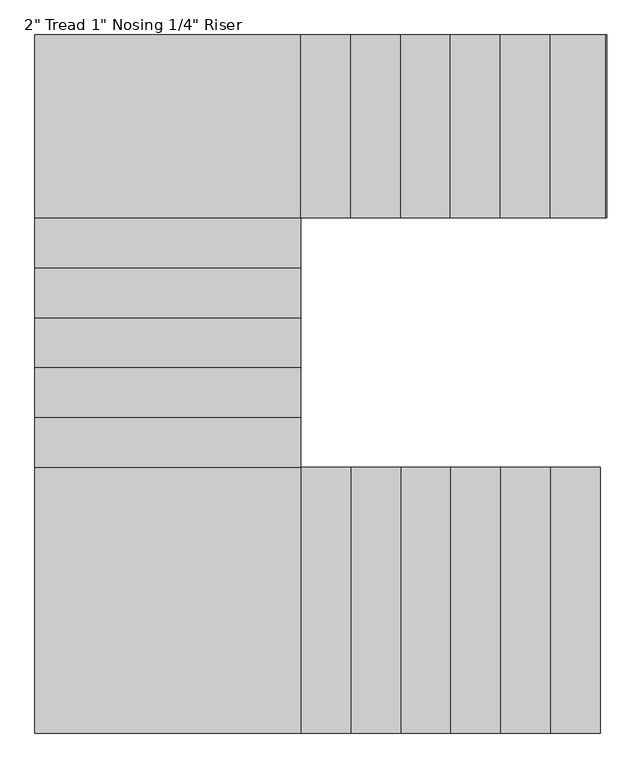
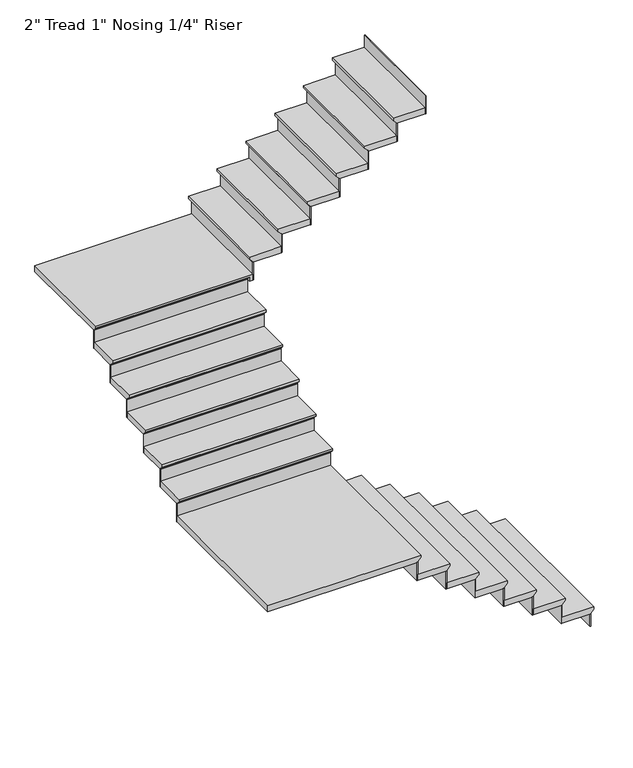
"""IFC4 building model written with IfcOpenShell, lengths in millimetres: stair flight geometry."""

from ifc_helpers import new_model, si_unit, origin, place, context, project, spatial, faceted_brep, source, transform, mapped, element, save


def stair_flight_3f57ae35(model_context):
    return source(origin(), model_context, "Body", "Brep", [
        faceted_brep([(-2515.2117403, -5163.0426559, 9582.15), (-2515.2117403, -5163.0426559, 9601.2), (-2515.2117403, -6382.2426559, 9601.2), (-2515.2117403, -6382.2426559, 9582.15), (-2540.6117403, -5163.0426559, 9556.75), (-2540.6117403, -6382.2426559, 9556.75), (-2769.2117403, -5163.0426559, 9601.2), (-2769.2117403, -6382.2426559, 9601.2), (-2540.6117403, -6382.2426559, 9550.4), (-2769.2117403, -6382.2426559, 9550.4), (-2769.2117403, -5163.0426559, 9550.4), (-2540.6117403, -5163.0426559, 9550.4)], [[[0, 1, 2, 3]], [[4, 0, 3, 5]], [[2, 1, 6, 7]], [[8, 9, 10, 11]], [[2, 7, 9, 8, 5, 3]], [[8, 11, 4, 5]], [[6, 1, 0, 4, 11, 10]], [[7, 6, 10, 9]]]),
        faceted_brep([(-2540.6117403, -5163.0426559, 9550.4), (-2540.6117403, -5163.0426559, 9448.8), (-2546.9617403, -5163.0426559, 9448.8), (-2546.9617403, -5163.0426559, 9550.4), (-2540.6117403, -6382.2426559, 9550.4), (-2546.9617403, -6382.2426559, 9550.4), (-2546.9617403, -6382.2426559, 9448.8), (-2540.6117403, -6382.2426559, 9448.8)], [[[0, 1, 2, 3]], [[4, 5, 6, 7]], [[1, 0, 4, 7]], [[2, 1, 7, 6]], [[3, 2, 6, 5]], [[0, 3, 5, 4]]]),
        faceted_brep([(-2769.2117403, -5163.0426559, 9702.8), (-2769.2117403, -5163.0426559, 9550.4), (-2775.5617403, -5163.0426559, 9550.4), (-2775.5617403, -5163.0426559, 9702.8), (-2769.2117403, -6382.2426559, 9702.8), (-2775.5617403, -6382.2426559, 9702.8), (-2775.5617403, -6382.2426559, 9550.4), (-2769.2117403, -6382.2426559, 9550.4)], [[[0, 1, 2, 3]], [[4, 5, 6, 7]], [[1, 0, 4, 7]], [[2, 1, 7, 6]], [[3, 2, 6, 5]], [[0, 3, 5, 4]]]),
        faceted_brep([(-2743.8117403, -6382.2426559, 9753.6), (-2743.8117403, -5163.0426559, 9753.6), (-2997.8117403, -5163.0426559, 9753.6), (-2997.8117403, -6382.2426559, 9753.6), (-2769.2117403, -6382.2426559, 9702.8), (-2997.8117403, -6382.2426559, 9702.8), (-2997.8117403, -5163.0426559, 9702.8), (-2769.2117403, -5163.0426559, 9702.8), (-2769.2117403, -6382.2426559, 9709.15), (-2743.8117403, -6382.2426559, 9734.55), (-2769.2117403, -5163.0426559, 9709.15), (-2743.8117403, -5163.0426559, 9734.55)], [[[0, 1, 2, 3]], [[4, 5, 6, 7]], [[0, 3, 5, 4, 8, 9]], [[4, 7, 10, 8]], [[2, 1, 11, 10, 7, 6]], [[3, 2, 6, 5]], [[11, 1, 0, 9]], [[10, 11, 9, 8]]]),
        faceted_brep([(-2997.8117403, -5163.0426559, 9855.2), (-2997.8117403, -5163.0426559, 9702.8), (-3004.1617403, -5163.0426559, 9702.8), (-3004.1617403, -5163.0426559, 9855.2), (-2997.8117403, -6382.2426559, 9855.2), (-3004.1617403, -6382.2426559, 9855.2), (-3004.1617403, -6382.2426559, 9702.8), (-2997.8117403, -6382.2426559, 9702.8)], [[[0, 1, 2, 3]], [[4, 5, 6, 7]], [[1, 0, 4, 7]], [[2, 1, 7, 6]], [[3, 2, 6, 5]], [[0, 3, 5, 4]]]),
        faceted_brep([(-2972.4117403, -6382.2426559, 9906.0), (-2972.4117403, -5163.0426559, 9906.0), (-3226.4117403, -5163.0426559, 9906.0), (-3226.4117403, -6382.2426559, 9906.0), (-2997.8117403, -6382.2426559, 9855.2), (-3226.4117403, -6382.2426559, 9855.2), (-3226.4117403, -5163.0426559, 9855.2), (-2997.8117403, -5163.0426559, 9855.2), (-2997.8117403, -6382.2426559, 9861.55), (-2972.4117403, -6382.2426559, 9886.95), (-2997.8117403, -5163.0426559, 9861.55), (-2972.4117403, -5163.0426559, 9886.95)], [[[0, 1, 2, 3]], [[4, 5, 6, 7]], [[0, 3, 5, 4, 8, 9]], [[4, 7, 10, 8]], [[2, 1, 11, 10, 7, 6]], [[3, 2, 6, 5]], [[11, 1, 0, 9]], [[10, 11, 9, 8]]]),
        faceted_brep([(-3226.4117403, -5163.0426559, 10007.6), (-3226.4117403, -5163.0426559, 9855.2), (-3232.7617403, -5163.0426559, 9855.2), (-3232.7617403, -5163.0426559, 10007.6), (-3226.4117403, -6382.2426559, 10007.6), (-3232.7617403, -6382.2426559, 10007.6), (-3232.7617403, -6382.2426559, 9855.2), (-3226.4117403, -6382.2426559, 9855.2)], [[[0, 1, 2, 3]], [[4, 5, 6, 7]], [[1, 0, 4, 7]], [[2, 1, 7, 6]], [[3, 2, 6, 5]], [[0, 3, 5, 4]]]),
        faceted_brep([(-3201.0117403, -6382.2426559, 10058.4), (-3201.0117403, -5163.0426559, 10058.4), (-3455.0117403, -5163.0426559, 10058.4), (-3455.0117403, -6382.2426559, 10058.4), (-3226.4117403, -6382.2426559, 10007.6), (-3455.0117403, -6382.2426559, 10007.6), (-3455.0117403, -5163.0426559, 10007.6), (-3226.4117403, -5163.0426559, 10007.6), (-3226.4117403, -6382.2426559, 10013.95), (-3201.0117403, -6382.2426559, 10039.35), (-3226.4117403, -5163.0426559, 10013.95), (-3201.0117403, -5163.0426559, 10039.35)], [[[0, 1, 2, 3]], [[4, 5, 6, 7]], [[0, 3, 5, 4, 8, 9]], [[4, 7, 10, 8]], [[2, 1, 11, 10, 7, 6]], [[3, 2, 6, 5]], [[11, 1, 0, 9]], [[10, 11, 9, 8]]]),
        faceted_brep([(-3455.0117403, -5163.0426559, 10160.0), (-3455.0117403, -5163.0426559, 10007.6), (-3461.3617403, -5163.0426559, 10007.6), (-3461.3617403, -5163.0426559, 10160.0), (-3455.0117403, -6382.2426559, 10160.0), (-3461.3617403, -6382.2426559, 10160.0), (-3461.3617403, -6382.2426559, 10007.6), (-3455.0117403, -6382.2426559, 10007.6)], [[[0, 1, 2, 3]], [[4, 5, 6, 7]], [[1, 0, 4, 7]], [[2, 1, 7, 6]], [[3, 2, 6, 5]], [[0, 3, 5, 4]]]),
        faceted_brep([(-3429.6117403, -6382.2426559, 10210.8), (-3429.6117403, -5163.0426559, 10210.8), (-3683.6117403, -5163.0426559, 10210.8), (-3683.6117403, -6382.2426559, 10210.8), (-3455.0117403, -6382.2426559, 10160.0), (-3683.6117403, -6382.2426559, 10160.0), (-3683.6117403, -5163.0426559, 10160.0), (-3455.0117403, -5163.0426559, 10160.0), (-3455.0117403, -6382.2426559, 10166.35), (-3429.6117403, -6382.2426559, 10191.75), (-3455.0117403, -5163.0426559, 10166.35), (-3429.6117403, -5163.0426559, 10191.75)], [[[0, 1, 2, 3]], [[4, 5, 6, 7]], [[0, 3, 5, 4, 8, 9]], [[4, 7, 10, 8]], [[2, 1, 11, 10, 7, 6]], [[3, 2, 6, 5]], [[11, 1, 0, 9]], [[10, 11, 9, 8]]]),
        faceted_brep([(-3683.6117403, -5163.0426559, 10312.4), (-3683.6117403, -5163.0426559, 10160.0), (-3689.9617403, -5163.0426559, 10160.0), (-3689.9617403, -5163.0426559, 10312.4), (-3683.6117403, -6382.2426559, 10312.4), (-3689.9617403, -6382.2426559, 10312.4), (-3689.9617403, -6382.2426559, 10160.0), (-3683.6117403, -6382.2426559, 10160.0)], [[[0, 1, 2, 3]], [[4, 5, 6, 7]], [[1, 0, 4, 7]], [[2, 1, 7, 6]], [[3, 2, 6, 5]], [[0, 3, 5, 4]]]),
        faceted_brep([(-3658.2117403, -6382.2426559, 10363.2), (-3658.2117403, -5163.0426559, 10363.2), (-3912.2117403, -5163.0426559, 10363.2), (-3912.2117403, -6382.2426559, 10363.2), (-3683.6117403, -6382.2426559, 10312.4), (-3912.2117403, -6382.2426559, 10312.4), (-3912.2117403, -5163.0426559, 10312.4), (-3683.6117403, -5163.0426559, 10312.4), (-3683.6117403, -6382.2426559, 10318.75), (-3658.2117403, -6382.2426559, 10344.15), (-3683.6117403, -5163.0426559, 10318.75), (-3658.2117403, -5163.0426559, 10344.15)], [[[0, 1, 2, 3]], [[4, 5, 6, 7]], [[0, 3, 5, 4, 8, 9]], [[4, 7, 10, 8]], [[2, 1, 11, 10, 7, 6]], [[3, 2, 6, 5]], [[11, 1, 0, 9]], [[10, 11, 9, 8]]]),
        faceted_brep([(-3912.2117403, -5163.0426559, 10464.8), (-3912.2117403, -5163.0426559, 10312.4), (-3918.5617403, -5163.0426559, 10312.4), (-3918.5617403, -5163.0426559, 10464.8), (-3912.2117403, -6382.2426559, 10464.8), (-3918.5617403, -6382.2426559, 10464.8), (-3918.5617403, -6382.2426559, 10312.4), (-3912.2117403, -6382.2426559, 10312.4)], [[[0, 1, 2, 3]], [[4, 5, 6, 7]], [[1, 0, 4, 7]], [[2, 1, 7, 6]], [[3, 2, 6, 5]], [[0, 3, 5, 4]]]),
        faceted_brep([(-5106.0117403, -5137.6426559, 10515.6), (-5106.0117403, -6382.2426559, 10515.6), (-3886.8117403, -6382.2426559, 10515.6), (-3886.8117403, -5137.6426559, 10515.6), (-5106.0117403, -6382.2426559, 10464.8), (-5106.0117403, -5137.6426559, 10464.8), (-3886.8117403, -5137.6426559, 10464.8), (-3886.8117403, -5163.0426559, 10464.8), (-3912.2117403, -5163.0426559, 10464.8), (-3912.2117403, -6382.2426559, 10464.8), (-3912.2117403, -6382.2426559, 10471.15), (-3886.8117403, -6382.2426559, 10496.55), (-3912.2117403, -5163.0426559, 10471.15), (-3886.8117403, -5163.0426559, 10496.55)], [[[0, 1, 2, 3]], [[4, 5, 6, 7, 8, 9]], [[1, 0, 5, 4]], [[2, 1, 4, 9, 10, 11]], [[9, 8, 12, 10]], [[8, 7, 13, 12]], [[3, 2, 11, 13, 7, 6]], [[0, 3, 6, 5]], [[11, 10, 12, 13]]]),
        faceted_brep([(-3886.8117403, -5137.6426559, 10617.2), (-3886.8117403, -5137.6426559, 10464.8), (-3886.8117403, -5131.2926559, 10464.8), (-3886.8117403, -5131.2926559, 10617.2), (-5106.0117403, -5137.6426559, 10617.2), (-5106.0117403, -5131.2926559, 10617.2), (-5106.0117403, -5131.2926559, 10464.8), (-5106.0117403, -5137.6426559, 10464.8)], [[[0, 1, 2, 3]], [[4, 5, 6, 7]], [[1, 0, 4, 7]], [[2, 1, 7, 6]], [[3, 2, 6, 5]], [[0, 3, 5, 4]]]),
        faceted_brep([(-5106.0117403, -5163.0426559, 10668.0), (-3886.8117403, -5163.0426559, 10668.0), (-3886.8117403, -4909.0426559, 10668.0), (-5106.0117403, -4909.0426559, 10668.0), (-5106.0117403, -5137.6426559, 10617.2), (-5106.0117403, -4909.0426559, 10617.2), (-3886.8117403, -4909.0426559, 10617.2), (-3886.8117403, -5137.6426559, 10617.2), (-5106.0117403, -5137.6426559, 10623.55), (-5106.0117403, -5163.0426559, 10648.95), (-3886.8117403, -5137.6426559, 10623.55), (-3886.8117403, -5163.0426559, 10648.95)], [[[0, 1, 2, 3]], [[4, 5, 6, 7]], [[0, 3, 5, 4, 8, 9]], [[4, 7, 10, 8]], [[2, 1, 11, 10, 7, 6]], [[3, 2, 6, 5]], [[11, 1, 0, 9]], [[10, 11, 9, 8]]]),
        faceted_brep([(-3886.8117403, -4909.0426559, 10769.6), (-3886.8117403, -4909.0426559, 10617.2), (-3886.8117403, -4902.6926559, 10617.2), (-3886.8117403, -4902.6926559, 10769.6), (-5106.0117403, -4909.0426559, 10769.6), (-5106.0117403, -4902.6926559, 10769.6), (-5106.0117403, -4902.6926559, 10617.2), (-5106.0117403, -4909.0426559, 10617.2)], [[[0, 1, 2, 3]], [[4, 5, 6, 7]], [[1, 0, 4, 7]], [[2, 1, 7, 6]], [[3, 2, 6, 5]], [[0, 3, 5, 4]]]),
        faceted_brep([(-5106.0117403, -4934.4426559, 10820.4), (-3886.8117403, -4934.4426559, 10820.4), (-3886.8117403, -4680.4426559, 10820.4), (-5106.0117403, -4680.4426559, 10820.4), (-5106.0117403, -4909.0426559, 10769.6), (-5106.0117403, -4680.4426559, 10769.6), (-3886.8117403, -4680.4426559, 10769.6), (-3886.8117403, -4909.0426559, 10769.6), (-5106.0117403, -4909.0426559, 10775.95), (-5106.0117403, -4934.4426559, 10801.35), (-3886.8117403, -4909.0426559, 10775.95), (-3886.8117403, -4934.4426559, 10801.35)], [[[0, 1, 2, 3]], [[4, 5, 6, 7]], [[0, 3, 5, 4, 8, 9]], [[4, 7, 10, 8]], [[2, 1, 11, 10, 7, 6]], [[3, 2, 6, 5]], [[11, 1, 0, 9]], [[10, 11, 9, 8]]]),
        faceted_brep([(-3886.8117403, -4680.4426559, 10922.0), (-3886.8117403, -4680.4426559, 10769.6), (-3886.8117403, -4674.0926559, 10769.6), (-3886.8117403, -4674.0926559, 10922.0), (-5106.0117403, -4680.4426559, 10922.0), (-5106.0117403, -4674.0926559, 10922.0), (-5106.0117403, -4674.0926559, 10769.6), (-5106.0117403, -4680.4426559, 10769.6)], [[[0, 1, 2, 3]], [[4, 5, 6, 7]], [[1, 0, 4, 7]], [[2, 1, 7, 6]], [[3, 2, 6, 5]], [[0, 3, 5, 4]]]),
        faceted_brep([(-5106.0117403, -4705.8426559, 10972.8), (-3886.8117403, -4705.8426559, 10972.8), (-3886.8117403, -4451.8426559, 10972.8), (-5106.0117403, -4451.8426559, 10972.8), (-5106.0117403, -4680.4426559, 10922.0), (-5106.0117403, -4451.8426559, 10922.0), (-3886.8117403, -4451.8426559, 10922.0), (-3886.8117403, -4680.4426559, 10922.0), (-5106.0117403, -4680.4426559, 10928.35), (-5106.0117403, -4705.8426559, 10953.75), (-3886.8117403, -4680.4426559, 10928.35), (-3886.8117403, -4705.8426559, 10953.75)], [[[0, 1, 2, 3]], [[4, 5, 6, 7]], [[0, 3, 5, 4, 8, 9]], [[4, 7, 10, 8]], [[2, 1, 11, 10, 7, 6]], [[3, 2, 6, 5]], [[11, 1, 0, 9]], [[10, 11, 9, 8]]]),
        faceted_brep([(-3886.8117403, -4451.8426559, 11074.4), (-3886.8117403, -4451.8426559, 10922.0), (-3886.8117403, -4445.4926559, 10922.0), (-3886.8117403, -4445.4926559, 11074.4), (-5106.0117403, -4451.8426559, 11074.4), (-5106.0117403, -4445.4926559, 11074.4), (-5106.0117403, -4445.4926559, 10922.0), (-5106.0117403, -4451.8426559, 10922.0)], [[[0, 1, 2, 3]], [[4, 5, 6, 7]], [[1, 0, 4, 7]], [[2, 1, 7, 6]], [[3, 2, 6, 5]], [[0, 3, 5, 4]]]),
        faceted_brep([(-5106.0117403, -4477.2426559, 11125.2), (-3886.8117403, -4477.2426559, 11125.2), (-3886.8117403, -4223.2426559, 11125.2), (-5106.0117403, -4223.2426559, 11125.2), (-5106.0117403, -4451.8426559, 11074.4), (-5106.0117403, -4223.2426559, 11074.4), (-3886.8117403, -4223.2426559, 11074.4), (-3886.8117403, -4451.8426559, 11074.4), (-5106.0117403, -4451.8426559, 11080.75), (-5106.0117403, -4477.2426559, 11106.15), (-3886.8117403, -4451.8426559, 11080.75), (-3886.8117403, -4477.2426559, 11106.15)], [[[0, 1, 2, 3]], [[4, 5, 6, 7]], [[0, 3, 5, 4, 8, 9]], [[4, 7, 10, 8]], [[2, 1, 11, 10, 7, 6]], [[3, 2, 6, 5]], [[11, 1, 0, 9]], [[10, 11, 9, 8]]]),
        faceted_brep([(-3886.8117403, -4223.2426559, 11226.8), (-3886.8117403, -4223.2426559, 11074.4), (-3886.8117403, -4216.8926559, 11074.4), (-3886.8117403, -4216.8926559, 11226.8), (-5106.0117403, -4223.2426559, 11226.8), (-5106.0117403, -4216.8926559, 11226.8), (-5106.0117403, -4216.8926559, 11074.4), (-5106.0117403, -4223.2426559, 11074.4)], [[[0, 1, 2, 3]], [[4, 5, 6, 7]], [[1, 0, 4, 7]], [[2, 1, 7, 6]], [[3, 2, 6, 5]], [[0, 3, 5, 4]]]),
        faceted_brep([(-5106.0117403, -4248.6426559, 11277.6), (-3886.8117403, -4248.6426559, 11277.6), (-3886.8117403, -3994.6426559, 11277.6), (-5106.0117403, -3994.6426559, 11277.6), (-5106.0117403, -4223.2426559, 11226.8), (-5106.0117403, -3994.6426559, 11226.8), (-3886.8117403, -3994.6426559, 11226.8), (-3886.8117403, -4223.2426559, 11226.8), (-5106.0117403, -4223.2426559, 11233.15), (-5106.0117403, -4248.6426559, 11258.55), (-3886.8117403, -4223.2426559, 11233.15), (-3886.8117403, -4248.6426559, 11258.55)], [[[0, 1, 2, 3]], [[4, 5, 6, 7]], [[0, 3, 5, 4, 8, 9]], [[4, 7, 10, 8]], [[2, 1, 11, 10, 7, 6]], [[3, 2, 6, 5]], [[11, 1, 0, 9]], [[10, 11, 9, 8]]]),
        faceted_brep([(-3886.8117403, -3994.6426559, 11379.2), (-3886.8117403, -3994.6426559, 11226.8), (-3886.8117403, -3988.2926559, 11226.8), (-3886.8117403, -3988.2926559, 11379.2), (-5106.0117403, -3994.6426559, 11379.2), (-5106.0117403, -3988.2926559, 11379.2), (-5106.0117403, -3988.2926559, 11226.8), (-5106.0117403, -3994.6426559, 11226.8)], [[[0, 1, 2, 3]], [[4, 5, 6, 7]], [[1, 0, 4, 7]], [[2, 1, 7, 6]], [[3, 2, 6, 5]], [[0, 3, 5, 4]]]),
        faceted_brep([(-3861.4117403, -3181.8426559, 11430.0), (-5106.0117403, -3181.8426559, 11430.0), (-5106.0117403, -4020.0426559, 11430.0), (-3861.4117403, -4020.0426559, 11430.0), (-5106.0117403, -3181.8426559, 11379.2), (-3861.4117403, -3181.8426559, 11379.2), (-3861.4117403, -4020.0426559, 11379.2), (-3886.8117403, -4020.0426559, 11379.2), (-3886.8117403, -3994.6426559, 11379.2), (-5106.0117403, -3994.6426559, 11379.2), (-5106.0117403, -3994.6426559, 11385.55), (-5106.0117403, -4020.0426559, 11410.95), (-3886.8117403, -3994.6426559, 11385.55), (-3886.8117403, -4020.0426559, 11410.95)], [[[0, 1, 2, 3]], [[4, 5, 6, 7, 8, 9]], [[1, 0, 5, 4]], [[2, 1, 4, 9, 10, 11]], [[9, 8, 12, 10]], [[8, 7, 13, 12]], [[3, 2, 11, 13, 7, 6]], [[0, 3, 6, 5]], [[11, 10, 12, 13]]]),
        faceted_brep([(-3861.4117403, -4020.0426559, 11531.6), (-3861.4117403, -4020.0426559, 11379.2), (-3855.0617403, -4020.0426559, 11379.2), (-3855.0617403, -4020.0426559, 11531.6), (-3861.4117403, -3181.8426559, 11531.6), (-3855.0617403, -3181.8426559, 11531.6), (-3855.0617403, -3181.8426559, 11379.2), (-3861.4117403, -3181.8426559, 11379.2)], [[[0, 1, 2, 3]], [[4, 5, 6, 7]], [[1, 0, 4, 7]], [[2, 1, 7, 6]], [[3, 2, 6, 5]], [[0, 3, 5, 4]]]),
        faceted_brep([(-3886.8117403, -3181.8426559, 11582.4), (-3886.8117403, -4020.0426559, 11582.4), (-3632.8117403, -4020.0426559, 11582.4), (-3632.8117403, -3181.8426559, 11582.4), (-3861.4117403, -3181.8426559, 11531.6), (-3632.8117403, -3181.8426559, 11531.6), (-3632.8117403, -4020.0426559, 11531.6), (-3861.4117403, -4020.0426559, 11531.6), (-3861.4117403, -3181.8426559, 11537.95), (-3886.8117403, -3181.8426559, 11563.35), (-3861.4117403, -4020.0426559, 11537.95), (-3886.8117403, -4020.0426559, 11563.35)], [[[0, 1, 2, 3]], [[4, 5, 6, 7]], [[0, 3, 5, 4, 8, 9]], [[4, 7, 10, 8]], [[2, 1, 11, 10, 7, 6]], [[3, 2, 6, 5]], [[11, 1, 0, 9]], [[10, 11, 9, 8]]]),
        faceted_brep([(-3632.8117403, -4020.0426559, 11684.0), (-3632.8117403, -4020.0426559, 11531.6), (-3626.4617403, -4020.0426559, 11531.6), (-3626.4617403, -4020.0426559, 11684.0), (-3632.8117403, -3181.8426559, 11684.0), (-3626.4617403, -3181.8426559, 11684.0), (-3626.4617403, -3181.8426559, 11531.6), (-3632.8117403, -3181.8426559, 11531.6)], [[[0, 1, 2, 3]], [[4, 5, 6, 7]], [[1, 0, 4, 7]], [[2, 1, 7, 6]], [[3, 2, 6, 5]], [[0, 3, 5, 4]]]),
        faceted_brep([(-3658.2117403, -3181.8426559, 11734.8), (-3658.2117403, -4020.0426559, 11734.8), (-3404.2117403, -4020.0426559, 11734.8), (-3404.2117403, -3181.8426559, 11734.8), (-3632.8117403, -3181.8426559, 11684.0), (-3404.2117403, -3181.8426559, 11684.0), (-3404.2117403, -4020.0426559, 11684.0), (-3632.8117403, -4020.0426559, 11684.0), (-3632.8117403, -3181.8426559, 11690.35), (-3658.2117403, -3181.8426559, 11715.75), (-3632.8117403, -4020.0426559, 11690.35), (-3658.2117403, -4020.0426559, 11715.75)], [[[0, 1, 2, 3]], [[4, 5, 6, 7]], [[0, 3, 5, 4, 8, 9]], [[4, 7, 10, 8]], [[2, 1, 11, 10, 7, 6]], [[3, 2, 6, 5]], [[11, 1, 0, 9]], [[10, 11, 9, 8]]]),
        faceted_brep([(-3404.2117403, -4020.0426559, 11836.4), (-3404.2117403, -4020.0426559, 11684.0), (-3397.8617403, -4020.0426559, 11684.0), (-3397.8617403, -4020.0426559, 11836.4), (-3404.2117403, -3181.8426559, 11836.4), (-3397.8617403, -3181.8426559, 11836.4), (-3397.8617403, -3181.8426559, 11684.0), (-3404.2117403, -3181.8426559, 11684.0)], [[[0, 1, 2, 3]], [[4, 5, 6, 7]], [[1, 0, 4, 7]], [[2, 1, 7, 6]], [[3, 2, 6, 5]], [[0, 3, 5, 4]]]),
        faceted_brep([(-3429.6117403, -3181.8426559, 11887.2), (-3429.6117403, -4020.0426559, 11887.2), (-3175.6117403, -4020.0426559, 11887.2), (-3175.6117403, -3181.8426559, 11887.2), (-3404.2117403, -3181.8426559, 11836.4), (-3175.6117403, -3181.8426559, 11836.4), (-3175.6117403, -4020.0426559, 11836.4), (-3404.2117403, -4020.0426559, 11836.4), (-3404.2117403, -3181.8426559, 11842.75), (-3429.6117403, -3181.8426559, 11868.15), (-3404.2117403, -4020.0426559, 11842.75), (-3429.6117403, -4020.0426559, 11868.15)], [[[0, 1, 2, 3]], [[4, 5, 6, 7]], [[0, 3, 5, 4, 8, 9]], [[4, 7, 10, 8]], [[2, 1, 11, 10, 7, 6]], [[3, 2, 6, 5]], [[11, 1, 0, 9]], [[10, 11, 9, 8]]]),
        faceted_brep([(-3175.6117403, -4020.0426559, 11988.8), (-3175.6117403, -4020.0426559, 11836.4), (-3169.2617403, -4020.0426559, 11836.4), (-3169.2617403, -4020.0426559, 11988.8), (-3175.6117403, -3181.8426559, 11988.8), (-3169.2617403, -3181.8426559, 11988.8), (-3169.2617403, -3181.8426559, 11836.4), (-3175.6117403, -3181.8426559, 11836.4)], [[[0, 1, 2, 3]], [[4, 5, 6, 7]], [[1, 0, 4, 7]], [[2, 1, 7, 6]], [[3, 2, 6, 5]], [[0, 3, 5, 4]]]),
        faceted_brep([(-3201.0117403, -3181.8426559, 12039.6), (-3201.0117403, -4020.0426559, 12039.6), (-2947.0117403, -4020.0426559, 12039.6), (-2947.0117403, -3181.8426559, 12039.6), (-3175.6117403, -3181.8426559, 11988.8), (-2947.0117403, -3181.8426559, 11988.8), (-2947.0117403, -4020.0426559, 11988.8), (-3175.6117403, -4020.0426559, 11988.8), (-3175.6117403, -3181.8426559, 11995.15), (-3201.0117403, -3181.8426559, 12020.55), (-3175.6117403, -4020.0426559, 11995.15), (-3201.0117403, -4020.0426559, 12020.55)], [[[0, 1, 2, 3]], [[4, 5, 6, 7]], [[0, 3, 5, 4, 8, 9]], [[4, 7, 10, 8]], [[2, 1, 11, 10, 7, 6]], [[3, 2, 6, 5]], [[11, 1, 0, 9]], [[10, 11, 9, 8]]]),
        faceted_brep([(-2947.0117403, -4020.0426559, 12141.2), (-2947.0117403, -4020.0426559, 11988.8), (-2940.6617403, -4020.0426559, 11988.8), (-2940.6617403, -4020.0426559, 12141.2), (-2947.0117403, -3181.8426559, 12141.2), (-2940.6617403, -3181.8426559, 12141.2), (-2940.6617403, -3181.8426559, 11988.8), (-2947.0117403, -3181.8426559, 11988.8)], [[[0, 1, 2, 3]], [[4, 5, 6, 7]], [[1, 0, 4, 7]], [[2, 1, 7, 6]], [[3, 2, 6, 5]], [[0, 3, 5, 4]]]),
        faceted_brep([(-2972.4117403, -3181.8426559, 12192.0), (-2972.4117403, -4020.0426559, 12192.0), (-2718.4117403, -4020.0426559, 12192.0), (-2718.4117403, -3181.8426559, 12192.0), (-2947.0117403, -3181.8426559, 12141.2), (-2718.4117403, -3181.8426559, 12141.2), (-2718.4117403, -4020.0426559, 12141.2), (-2947.0117403, -4020.0426559, 12141.2), (-2947.0117403, -3181.8426559, 12147.55), (-2972.4117403, -3181.8426559, 12172.95), (-2947.0117403, -4020.0426559, 12147.55), (-2972.4117403, -4020.0426559, 12172.95)], [[[0, 1, 2, 3]], [[4, 5, 6, 7]], [[0, 3, 5, 4, 8, 9]], [[4, 7, 10, 8]], [[2, 1, 11, 10, 7, 6]], [[3, 2, 6, 5]], [[11, 1, 0, 9]], [[10, 11, 9, 8]]]),
        faceted_brep([(-2718.4117403, -4020.0426559, 12293.6), (-2718.4117403, -4020.0426559, 12141.2), (-2712.0617403, -4020.0426559, 12141.2), (-2712.0617403, -4020.0426559, 12293.6), (-2718.4117403, -3181.8426559, 12293.6), (-2712.0617403, -3181.8426559, 12293.6), (-2712.0617403, -3181.8426559, 12141.2), (-2718.4117403, -3181.8426559, 12141.2)], [[[0, 1, 2, 3]], [[4, 5, 6, 7]], [[1, 0, 4, 7]], [[2, 1, 7, 6]], [[3, 2, 6, 5]], [[0, 3, 5, 4]]]),
        faceted_brep([(-2489.8117403, -4020.0426559, 12446.0), (-2489.8117403, -4020.0426559, 12293.6), (-2483.4617403, -4020.0426559, 12293.6), (-2483.4617403, -4020.0426559, 12446.0), (-2489.8117403, -3181.8426559, 12446.0), (-2483.4617403, -3181.8426559, 12446.0), (-2483.4617403, -3181.8426559, 12293.6), (-2489.8117403, -3181.8426559, 12293.6)], [[[0, 1, 2, 3]], [[4, 5, 6, 7]], [[1, 0, 4, 7]], [[2, 1, 7, 6]], [[3, 2, 6, 5]], [[0, 3, 5, 4]]]),
        faceted_brep([(-2743.8117403, -3181.8426559, 12344.4), (-2743.8117403, -4020.0426559, 12344.4), (-2489.8117403, -4020.0426559, 12344.4), (-2489.8117403, -3181.8426559, 12344.4), (-2718.4117403, -3181.8426559, 12293.6), (-2489.8117403, -3181.8426559, 12293.6), (-2489.8117403, -4020.0426559, 12293.6), (-2718.4117403, -4020.0426559, 12293.6), (-2718.4117403, -3181.8426559, 12299.95), (-2743.8117403, -3181.8426559, 12325.35), (-2718.4117403, -4020.0426559, 12299.95), (-2743.8117403, -4020.0426559, 12325.35)], [[[0, 1, 2, 3]], [[4, 5, 6, 7]], [[0, 3, 5, 4, 8, 9]], [[4, 7, 10, 8]], [[2, 1, 11, 10, 7, 6]], [[3, 2, 6, 5]], [[11, 1, 0, 9]], [[10, 11, 9, 8]]]),
    ])


if __name__ == "__main__":
    model = new_model("IFC4")
    model_context = context("Model", 3, world=origin())
    ifc_project = project(units=[si_unit("LENGTHUNIT", "METRE", prefix="MILLI")], contexts=[model_context])
    site = spatial("IfcSite", under=ifc_project)
    building = spatial("IfcBuilding", under=site)
    placement = place(None, origin())
    stair_flight_shape = stair_flight_3f57ae35(model_context)
    element("IfcStairFlight", 1, ObjectType="2\" Tread 1\" Nosing 1/4\" Riser", at=placement, inside=building, context=model_context, shape_type="MappedRepresentation", body=[
        mapped(stair_flight_shape, transform((0.0, 0.0, 0.0), x_axis=(1.0, 0.0, 0.0), y_axis=(0.0, 1.0, 0.0), z_axis=(0.0, 0.0, 1.0))),
    ])
    save(model, "model.ifc")

# Revit data of these elements
# Element 1 (IfcStairFlight, "2\" Tread 1\" Nosing 1/4\" Riser")
#   Materials on its faces: "Wood Planks"
# Materials
#   "Wood Planks": class "Wood", colour RGB 193 160 115, transparency 0, Description = "Physical material.", Cost = 0
